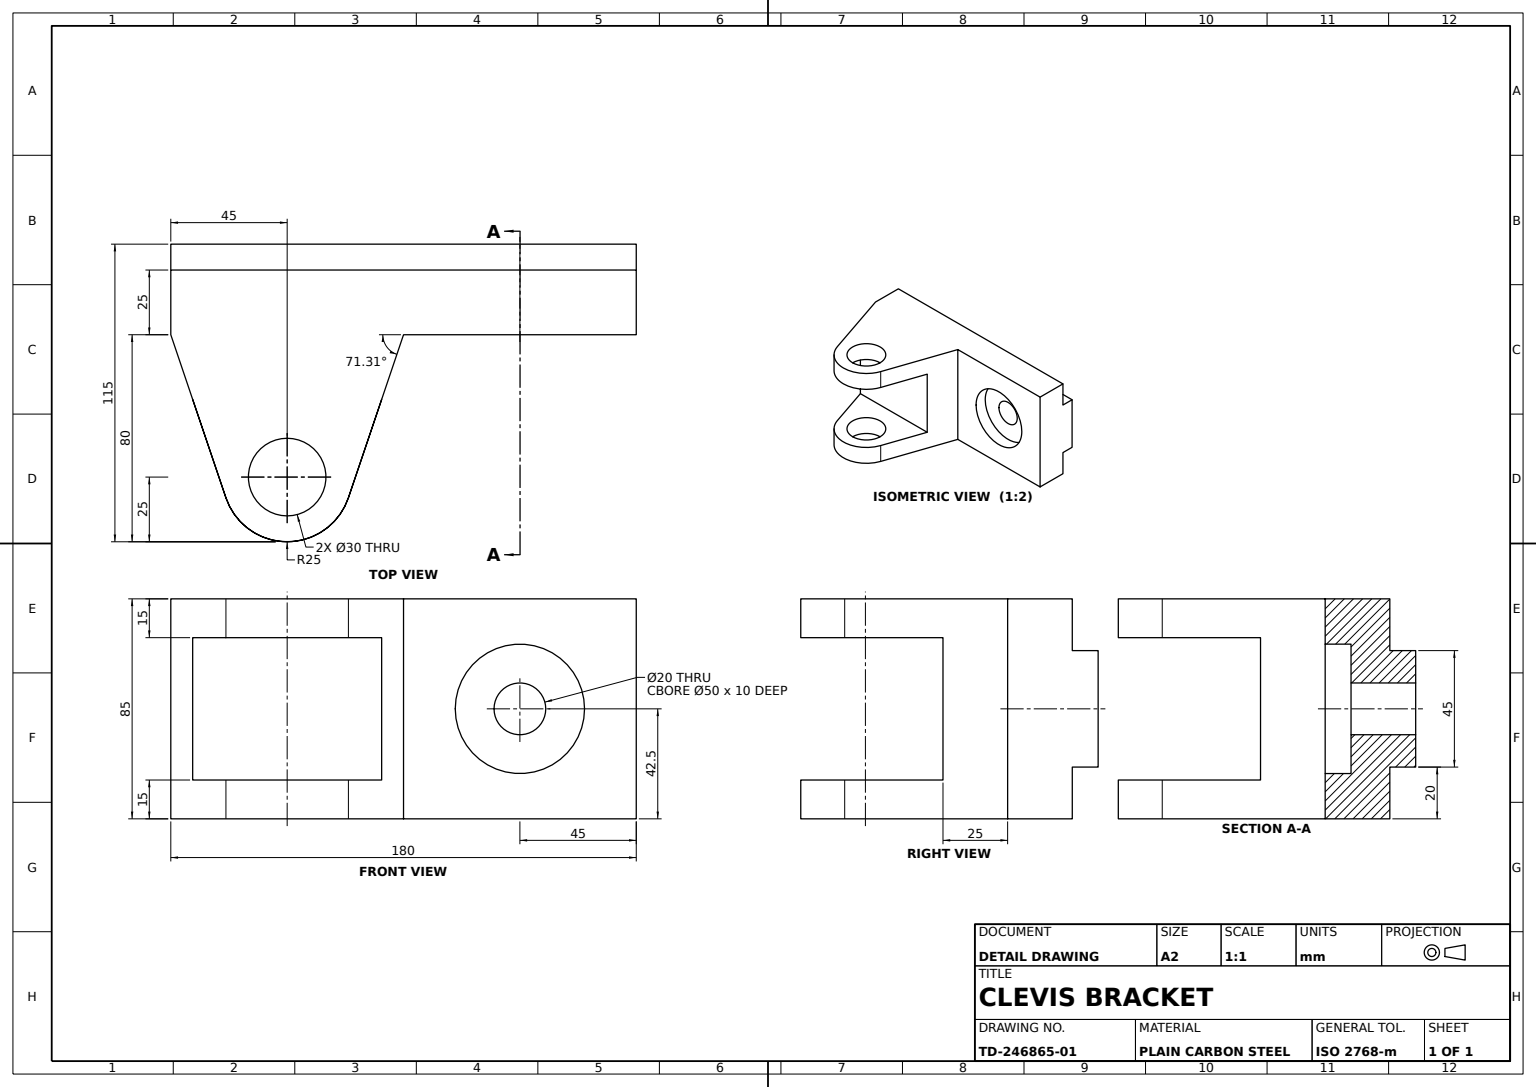
from build123d import *

# Parameters (mm, degrees)
BASE_PLATE_SKETCH_W   = 180
BASE_PLATE_SKETCH_H   = 85
BASE_PLATE_DEPTH      = 25
COUNTERBORE_SKETCH_R  = 25
COUNTERBORE_50_DEPTH  = 10
THROUGH_HOLE_SKETCH_R = 10
THROUGH_HOLE_20_DEPTH = 20
BACK_KEY_SKETCH_W     = 10
BACK_KEY_SKETCH_H     = 45
BACK_KEY_DEPTH        = 180
KEY_RELIEF_SKETCH_R   = 10
KEY_RELIEF_CUT_DEPTH  = 103.621878759
UPPER_LUG_SKETCH_R    = 15
UPPER_LUG_DEPTH       = 15
LOWER_START           = -15
LOWER_LUG_SKETCH_R    = 15
LOWER_LUG_DEPTH       = 15
LUG_WEB_SKETCH_W      = 90
LUG_WEB_SKETCH_H      = 55
LUG_WEB_DEPTH         = 25
WEB_CUT_A_DEPTH       = 156
WEB_CUT_B_DEPTH       = 156


with BuildPart() as part:
    # Base Plate Sketch → Base Plate (new body)
    with BuildSketch(Plane.XY):
        Rectangle(BASE_PLATE_SKETCH_W, BASE_PLATE_SKETCH_H)
    extrude(amount=BASE_PLATE_DEPTH)

    # Counterbore Sketch → Counterbore Ø50 (cut)
    with BuildSketch(Plane.XY.offset(25)):
        with Locations((45, 0)):
            Circle(COUNTERBORE_SKETCH_R)
    extrude(amount=-COUNTERBORE_50_DEPTH, mode=Mode.SUBTRACT)

    # Through Hole Sketch → Through Hole Ø20 (cut)
    with BuildSketch(Plane.XY.offset(15)):
        with Locations((45, 0)):
            Circle(THROUGH_HOLE_SKETCH_R)
    extrude(amount=-THROUGH_HOLE_20_DEPTH, mode=Mode.SUBTRACT)

    # Back Key Sketch → Back Key (add, through all)
    with BuildSketch(Plane.ZY.offset(90)):
        with Locations((-5, 0)):
            Rectangle(BACK_KEY_SKETCH_W, BACK_KEY_SKETCH_H)
    extrude(amount=-BACK_KEY_DEPTH)

    # Key Relief Sketch → Key Relief Cut (cut, through all)
    with BuildSketch(Plane.XY):
        with Locations((45, 0)):
            Circle(KEY_RELIEF_SKETCH_R)
    extrude(amount=-KEY_RELIEF_CUT_DEPTH, mode=Mode.SUBTRACT)

    # Upper Lug Sketch → Upper Lug (add)
    with BuildSketch(Plane.XZ.offset(42.5)):
        with BuildLine():
            Line((-68.681371492, 88.01203122), (-90, 25))
            Line((-90, 25), (0, 25))
            Line((0, 25), (-21.318628508, 88.01203122))
            ThreePointArc((-21.318628508, 88.01203122), (-45, 105), (-68.681371492, 88.01203122))
        make_face()
        with Locations(Location((-45, 80, 0), (0, 0, 270))):
            Circle(UPPER_LUG_SKETCH_R, mode=Mode.SUBTRACT)
    extrude(amount=-UPPER_LUG_DEPTH)

    # Lower Lug Sketch → Lower Lug (add)
    with BuildSketch(Plane(origin=(0, 42.5, 0), x_dir=(1, 0, 0), z_dir=(0, 1, 0)).offset(LOWER_START)):
        with BuildLine():
            Line((-90, -25), (-68.681371492, -88.01203122))
            ThreePointArc((-68.681371492, -88.01203122), (-45, -105), (-21.318628508, -88.01203122))
            Line((-21.318628508, -88.01203122), (0, -25))
            Line((0, -25), (-90, -25))
        make_face()
        with Locations(Location((-45, -80, 0), (0, 0, 90))):
            Circle(LOWER_LUG_SKETCH_R, mode=Mode.SUBTRACT)
    extrude(amount=LOWER_LUG_DEPTH)

    # Lug Web Sketch → Lug Web (add)
    with BuildSketch(Plane.XY.offset(25)):
        with Locations((-45, 0)):
            Rectangle(LUG_WEB_SKETCH_W, LUG_WEB_SKETCH_H)
    extrude(amount=LUG_WEB_DEPTH)

    # Web Cut A Sketch → Web Cut A (cut, through all)
    with BuildSketch(Plane(origin=(0, 27.5, 0), x_dir=(1, 0, 0), z_dir=(0, 1, 0))):
        Polygon((0, -25), (-8.458157948, -50), (0, -50), align=None)
    extrude(amount=-WEB_CUT_A_DEPTH, mode=Mode.SUBTRACT)

    # Web Cut B Sketch → Web Cut B (cut, through all)
    with BuildSketch(Plane.XZ.offset(27.5)):
        Polygon((-90, 25), (-81.541842052, 50), (-90, 50), align=None)
    extrude(amount=-WEB_CUT_B_DEPTH, mode=Mode.SUBTRACT)


solid = part.part
